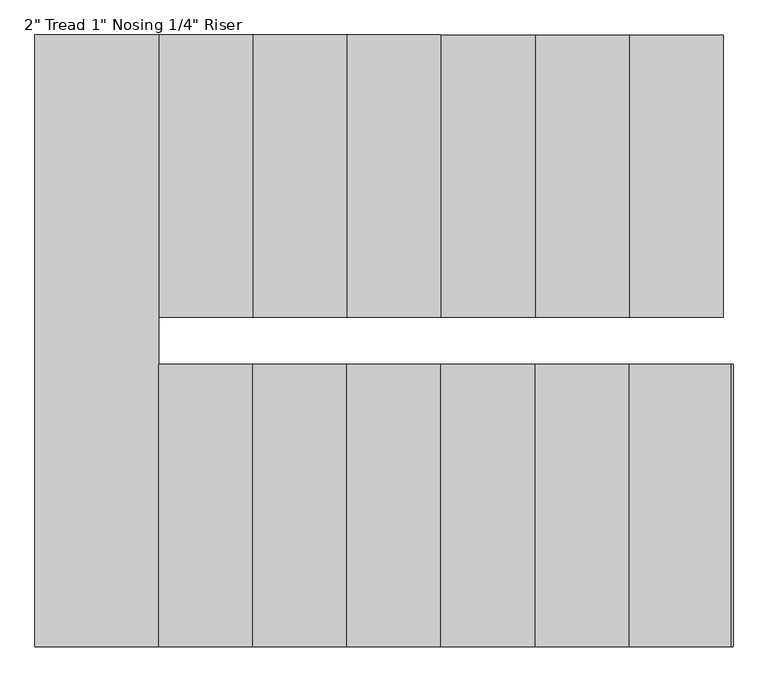
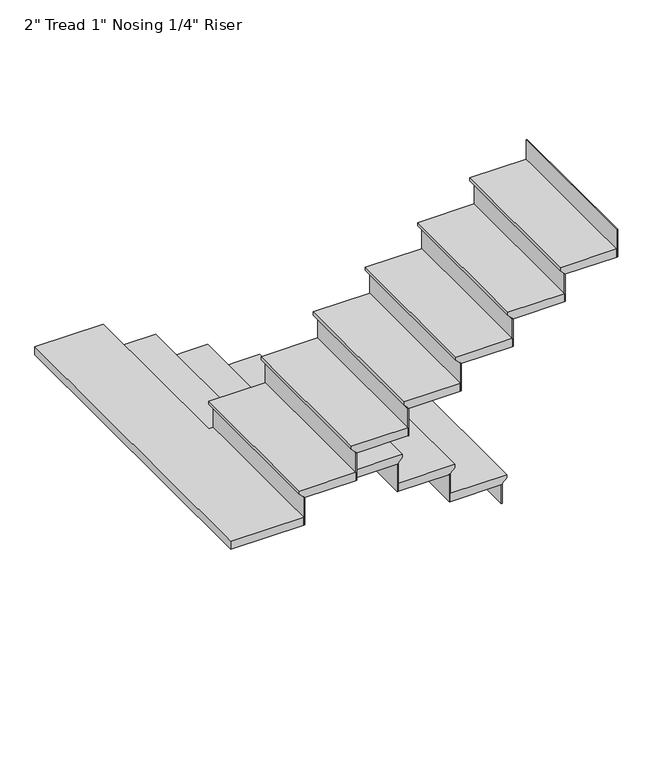
"""IFC4 building model written with IfcOpenShell, lengths in millimetres: stair flight geometry."""

from ifc_helpers import new_model, si_unit, origin, place, context, project, spatial, faceted_brep, source, transform, mapped, element, save


def stair_flight_ac649a0f(model_context):
    return source(origin(), model_context, "Body", "Brep", [
        faceted_brep([(3727.9146873, 3708.4, 9294.2833333), (3727.9146873, 3708.4, 9313.3333333), (3727.9146873, 2794.0, 9313.3333333), (3727.9146873, 2794.0, 9294.2833333), (3702.5146873, 3708.4, 9268.8833333), (3702.5146873, 2794.0, 9268.8833333), (3397.7146873, 3708.4, 9313.3333333), (3397.7146873, 2794.0, 9313.3333333), (3702.5146873, 2794.0, 9262.5333333), (3397.7146873, 2794.0, 9262.5333333), (3397.7146873, 3708.4, 9262.5333333), (3702.5146873, 3708.4, 9262.5333333)], [[[0, 1, 2, 3]], [[4, 0, 3, 5]], [[2, 1, 6, 7]], [[8, 9, 10, 11]], [[2, 7, 9, 8, 5, 3]], [[8, 11, 4, 5]], [[6, 1, 0, 4, 11, 10]], [[7, 6, 10, 9]]]),
        faceted_brep([(3702.5146873, 3708.4, 9262.5333333), (3702.5146873, 3708.4, 9144.0), (3696.1646873, 3708.4, 9144.0), (3696.1646873, 3708.4, 9262.5333333), (3702.5146873, 2794.0, 9262.5333333), (3696.1646873, 2794.0, 9262.5333333), (3696.1646873, 2794.0, 9144.0), (3702.5146873, 2794.0, 9144.0)], [[[0, 1, 2, 3]], [[4, 5, 6, 7]], [[1, 0, 4, 7]], [[2, 1, 7, 6]], [[3, 2, 6, 5]], [[0, 3, 5, 4]]]),
        faceted_brep([(3397.7146873, 3708.4, 9431.8666667), (3397.7146873, 3708.4, 9262.5333333), (3391.3646873, 3708.4, 9262.5333333), (3391.3646873, 3708.4, 9431.8666667), (3397.7146873, 2794.0, 9431.8666667), (3391.3646873, 2794.0, 9431.8666667), (3391.3646873, 2794.0, 9262.5333333), (3397.7146873, 2794.0, 9262.5333333)], [[[0, 1, 2, 3]], [[4, 5, 6, 7]], [[1, 0, 4, 7]], [[2, 1, 7, 6]], [[3, 2, 6, 5]], [[0, 3, 5, 4]]]),
        faceted_brep([(3423.1146873, 2794.0, 9482.6666667), (3423.1146873, 3708.4, 9482.6666667), (3092.9146873, 3708.4, 9482.6666667), (3092.9146873, 2794.0, 9482.6666667), (3397.7146873, 2794.0, 9431.8666667), (3092.9146873, 2794.0, 9431.8666667), (3092.9146873, 3708.4, 9431.8666667), (3397.7146873, 3708.4, 9431.8666667), (3397.7146873, 2794.0, 9438.2166667), (3423.1146873, 2794.0, 9463.6166667), (3397.7146873, 3708.4, 9438.2166667), (3423.1146873, 3708.4, 9463.6166667)], [[[0, 1, 2, 3]], [[4, 5, 6, 7]], [[0, 3, 5, 4, 8, 9]], [[4, 7, 10, 8]], [[2, 1, 11, 10, 7, 6]], [[3, 2, 6, 5]], [[11, 1, 0, 9]], [[10, 11, 9, 8]]]),
        faceted_brep([(3092.9146873, 3708.4, 9601.2), (3092.9146873, 3708.4, 9431.8666667), (3086.5646873, 3708.4, 9431.8666667), (3086.5646873, 3708.4, 9601.2), (3092.9146873, 2794.0, 9601.2), (3086.5646873, 2794.0, 9601.2), (3086.5646873, 2794.0, 9431.8666667), (3092.9146873, 2794.0, 9431.8666667)], [[[0, 1, 2, 3]], [[4, 5, 6, 7]], [[1, 0, 4, 7]], [[2, 1, 7, 6]], [[3, 2, 6, 5]], [[0, 3, 5, 4]]]),
        faceted_brep([(3118.3146873, 2794.0, 9652.0), (3118.3146873, 3708.4, 9652.0), (2788.1146873, 3708.4, 9652.0), (2788.1146873, 2794.0, 9652.0), (3092.9146873, 2794.0, 9601.2), (2788.1146873, 2794.0, 9601.2), (2788.1146873, 3708.4, 9601.2), (3092.9146873, 3708.4, 9601.2), (3092.9146873, 2794.0, 9607.55), (3118.3146873, 2794.0, 9632.95), (3092.9146873, 3708.4, 9607.55), (3118.3146873, 3708.4, 9632.95)], [[[0, 1, 2, 3]], [[4, 5, 6, 7]], [[0, 3, 5, 4, 8, 9]], [[4, 7, 10, 8]], [[2, 1, 11, 10, 7, 6]], [[3, 2, 6, 5]], [[11, 1, 0, 9]], [[10, 11, 9, 8]]]),
        faceted_brep([(2788.1146873, 3708.4, 9770.5333333), (2788.1146873, 3708.4, 9601.2), (2781.7646873, 3708.4, 9601.2), (2781.7646873, 3708.4, 9770.5333333), (2788.1146873, 2794.0, 9770.5333333), (2781.7646873, 2794.0, 9770.5333333), (2781.7646873, 2794.0, 9601.2), (2788.1146873, 2794.0, 9601.2)], [[[0, 1, 2, 3]], [[4, 5, 6, 7]], [[1, 0, 4, 7]], [[2, 1, 7, 6]], [[3, 2, 6, 5]], [[0, 3, 5, 4]]]),
        faceted_brep([(2813.5146873, 2794.0, 9821.3333333), (2813.5146873, 3708.4, 9821.3333333), (2483.3146873, 3708.4, 9821.3333333), (2483.3146873, 2794.0, 9821.3333333), (2788.1146873, 2794.0, 9770.5333333), (2483.3146873, 2794.0, 9770.5333333), (2483.3146873, 3708.4, 9770.5333333), (2788.1146873, 3708.4, 9770.5333333), (2788.1146873, 2794.0, 9776.8833333), (2813.5146873, 2794.0, 9802.2833333), (2788.1146873, 3708.4, 9776.8833333), (2813.5146873, 3708.4, 9802.2833333)], [[[0, 1, 2, 3]], [[4, 5, 6, 7]], [[0, 3, 5, 4, 8, 9]], [[4, 7, 10, 8]], [[2, 1, 11, 10, 7, 6]], [[3, 2, 6, 5]], [[11, 1, 0, 9]], [[10, 11, 9, 8]]]),
        faceted_brep([(2483.3146873, 3708.4, 9939.8666667), (2483.3146873, 3708.4, 9770.5333333), (2476.9646873, 3708.4, 9770.5333333), (2476.9646873, 3708.4, 9939.8666667), (2483.3146873, 2794.0, 9939.8666667), (2476.9646873, 2794.0, 9939.8666667), (2476.9646873, 2794.0, 9770.5333333), (2483.3146873, 2794.0, 9770.5333333)], [[[0, 1, 2, 3]], [[4, 5, 6, 7]], [[1, 0, 4, 7]], [[2, 1, 7, 6]], [[3, 2, 6, 5]], [[0, 3, 5, 4]]]),
        faceted_brep([(2508.7146873, 2794.0, 9990.6666667), (2508.7146873, 3708.4, 9990.6666667), (2178.5146873, 3708.4, 9990.6666667), (2178.5146873, 2794.0, 9990.6666667), (2483.3146873, 2794.0, 9939.8666667), (2178.5146873, 2794.0, 9939.8666667), (2178.5146873, 3708.4, 9939.8666667), (2483.3146873, 3708.4, 9939.8666667), (2483.3146873, 2794.0, 9946.2166667), (2508.7146873, 2794.0, 9971.6166667), (2483.3146873, 3708.4, 9946.2166667), (2508.7146873, 3708.4, 9971.6166667)], [[[0, 1, 2, 3]], [[4, 5, 6, 7]], [[0, 3, 5, 4, 8, 9]], [[4, 7, 10, 8]], [[2, 1, 11, 10, 7, 6]], [[3, 2, 6, 5]], [[11, 1, 0, 9]], [[10, 11, 9, 8]]]),
        faceted_brep([(2178.5146873, 3708.4, 10109.2), (2178.5146873, 3708.4, 9939.8666667), (2172.1646873, 3708.4, 9939.8666667), (2172.1646873, 3708.4, 10109.2), (2178.5146873, 2794.0, 10109.2), (2172.1646873, 2794.0, 10109.2), (2172.1646873, 2794.0, 9939.8666667), (2178.5146873, 2794.0, 9939.8666667)], [[[0, 1, 2, 3]], [[4, 5, 6, 7]], [[1, 0, 4, 7]], [[2, 1, 7, 6]], [[3, 2, 6, 5]], [[0, 3, 5, 4]]]),
        faceted_brep([(2203.9146873, 2794.0, 10160.0), (2203.9146873, 3708.4, 10160.0), (1873.7146873, 3708.4, 10160.0), (1873.7146873, 2794.0, 10160.0), (2178.5146873, 2794.0, 10109.2), (1873.7146873, 2794.0, 10109.2), (1873.7146873, 3708.4, 10109.2), (2178.5146873, 3708.4, 10109.2), (2178.5146873, 2794.0, 10115.55), (2203.9146873, 2794.0, 10140.95), (2178.5146873, 3708.4, 10115.55), (2203.9146873, 3708.4, 10140.95)], [[[0, 1, 2, 3]], [[4, 5, 6, 7]], [[0, 3, 5, 4, 8, 9]], [[4, 7, 10, 8]], [[2, 1, 11, 10, 7, 6]], [[3, 2, 6, 5]], [[11, 1, 0, 9]], [[10, 11, 9, 8]]]),
        faceted_brep([(1873.7146873, 3708.4, 10278.5333333), (1873.7146873, 3708.4, 10109.2), (1867.3646873, 3708.4, 10109.2), (1867.3646873, 3708.4, 10278.5333333), (1873.7146873, 2794.0, 10278.5333333), (1867.3646873, 2794.0, 10278.5333333), (1867.3646873, 2794.0, 10109.2), (1873.7146873, 2794.0, 10109.2)], [[[0, 1, 2, 3]], [[4, 5, 6, 7]], [[1, 0, 4, 7]], [[2, 1, 7, 6]], [[3, 2, 6, 5]], [[0, 3, 5, 4]]]),
        faceted_brep([(1924.5146873, 2641.6, 10329.3333333), (1899.1146873, 2641.6, 10329.3333333), (1899.1146873, 3708.4, 10329.3333333), (1498.6, 3708.4, 10329.3333333), (1498.6, 1727.2, 10329.3333333), (1924.5146873, 1727.2, 10329.3333333), (1899.1146873, 2641.6, 10278.5333333), (1924.5146873, 2641.6, 10278.5333333), (1924.5146873, 1727.2, 10278.5333333), (1498.6, 1727.2, 10278.5333333), (1498.6, 3708.4, 10278.5333333), (1873.7146873, 3708.4, 10278.5333333), (1873.7146873, 2794.0, 10278.5333333), (1899.1146873, 2794.0, 10278.5333333), (1899.1146873, 2794.0, 10310.2833333), (1899.1146873, 3708.4, 10310.2833333), (1873.7146873, 2794.0, 10284.8833333), (1873.7146873, 3708.4, 10284.8833333)], [[[0, 1, 2, 3, 4, 5]], [[6, 7, 8, 9, 10, 11, 12, 13]], [[1, 0, 7, 6]], [[2, 1, 6, 13, 14, 15]], [[13, 12, 16, 14]], [[12, 11, 17, 16]], [[3, 2, 15, 17, 11, 10]], [[4, 3, 10, 9]], [[5, 4, 9, 8]], [[0, 5, 8, 7]], [[17, 15, 14, 16]]]),
        faceted_brep([(1924.5146873, 1727.2, 10447.8666667), (1924.5146873, 1727.2, 10278.5333333), (1930.8646873, 1727.2, 10278.5333333), (1930.8646873, 1727.2, 10447.8666667), (1924.5146873, 2641.6, 10447.8666667), (1930.8646873, 2641.6, 10447.8666667), (1930.8646873, 2641.6, 10278.5333333), (1924.5146873, 2641.6, 10278.5333333)], [[[0, 1, 2, 3]], [[4, 5, 6, 7]], [[1, 0, 4, 7]], [[2, 1, 7, 6]], [[3, 2, 6, 5]], [[0, 3, 5, 4]]]),
        faceted_brep([(1899.1146873, 2641.6, 10498.6666667), (1899.1146873, 1727.2, 10498.6666667), (2229.3146873, 1727.2, 10498.6666667), (2229.3146873, 2641.6, 10498.6666667), (1924.5146873, 2641.6, 10447.8666667), (2229.3146873, 2641.6, 10447.8666667), (2229.3146873, 1727.2, 10447.8666667), (1924.5146873, 1727.2, 10447.8666667), (1924.5146873, 2641.6, 10454.2166667), (1899.1146873, 2641.6, 10479.6166667), (1924.5146873, 1727.2, 10454.2166667), (1899.1146873, 1727.2, 10479.6166667)], [[[0, 1, 2, 3]], [[4, 5, 6, 7]], [[0, 3, 5, 4, 8, 9]], [[4, 7, 10, 8]], [[2, 1, 11, 10, 7, 6]], [[3, 2, 6, 5]], [[11, 1, 0, 9]], [[10, 11, 9, 8]]]),
        faceted_brep([(2229.3146873, 1727.2, 10617.2), (2229.3146873, 1727.2, 10447.8666667), (2235.6646873, 1727.2, 10447.8666667), (2235.6646873, 1727.2, 10617.2), (2229.3146873, 2641.6, 10617.2), (2235.6646873, 2641.6, 10617.2), (2235.6646873, 2641.6, 10447.8666667), (2229.3146873, 2641.6, 10447.8666667)], [[[0, 1, 2, 3]], [[4, 5, 6, 7]], [[1, 0, 4, 7]], [[2, 1, 7, 6]], [[3, 2, 6, 5]], [[0, 3, 5, 4]]]),
        faceted_brep([(2203.9146873, 2641.6, 10668.0), (2203.9146873, 1727.2, 10668.0), (2534.1146873, 1727.2, 10668.0), (2534.1146873, 2641.6, 10668.0), (2229.3146873, 2641.6, 10617.2), (2534.1146873, 2641.6, 10617.2), (2534.1146873, 1727.2, 10617.2), (2229.3146873, 1727.2, 10617.2), (2229.3146873, 2641.6, 10623.55), (2203.9146873, 2641.6, 10648.95), (2229.3146873, 1727.2, 10623.55), (2203.9146873, 1727.2, 10648.95)], [[[0, 1, 2, 3]], [[4, 5, 6, 7]], [[0, 3, 5, 4, 8, 9]], [[4, 7, 10, 8]], [[2, 1, 11, 10, 7, 6]], [[3, 2, 6, 5]], [[11, 1, 0, 9]], [[10, 11, 9, 8]]]),
        faceted_brep([(2534.1146873, 1727.2, 10786.5333333), (2534.1146873, 1727.2, 10617.2), (2540.4646873, 1727.2, 10617.2), (2540.4646873, 1727.2, 10786.5333333), (2534.1146873, 2641.6, 10786.5333333), (2540.4646873, 2641.6, 10786.5333333), (2540.4646873, 2641.6, 10617.2), (2534.1146873, 2641.6, 10617.2)], [[[0, 1, 2, 3]], [[4, 5, 6, 7]], [[1, 0, 4, 7]], [[2, 1, 7, 6]], [[3, 2, 6, 5]], [[0, 3, 5, 4]]]),
        faceted_brep([(2508.7146873, 2641.6, 10837.3333333), (2508.7146873, 1727.2, 10837.3333333), (2838.9146873, 1727.2, 10837.3333333), (2838.9146873, 2641.6, 10837.3333333), (2534.1146873, 2641.6, 10786.5333333), (2838.9146873, 2641.6, 10786.5333333), (2838.9146873, 1727.2, 10786.5333333), (2534.1146873, 1727.2, 10786.5333333), (2534.1146873, 2641.6, 10792.8833333), (2508.7146873, 2641.6, 10818.2833333), (2534.1146873, 1727.2, 10792.8833333), (2508.7146873, 1727.2, 10818.2833333)], [[[0, 1, 2, 3]], [[4, 5, 6, 7]], [[0, 3, 5, 4, 8, 9]], [[4, 7, 10, 8]], [[2, 1, 11, 10, 7, 6]], [[3, 2, 6, 5]], [[11, 1, 0, 9]], [[10, 11, 9, 8]]]),
        faceted_brep([(2838.9146873, 1727.2, 10955.8666667), (2838.9146873, 1727.2, 10786.5333333), (2845.2646873, 1727.2, 10786.5333333), (2845.2646873, 1727.2, 10955.8666667), (2838.9146873, 2641.6, 10955.8666667), (2845.2646873, 2641.6, 10955.8666667), (2845.2646873, 2641.6, 10786.5333333), (2838.9146873, 2641.6, 10786.5333333)], [[[0, 1, 2, 3]], [[4, 5, 6, 7]], [[1, 0, 4, 7]], [[2, 1, 7, 6]], [[3, 2, 6, 5]], [[0, 3, 5, 4]]]),
        faceted_brep([(2813.5146873, 2641.6, 11006.6666667), (2813.5146873, 1727.2, 11006.6666667), (3143.7146873, 1727.2, 11006.6666667), (3143.7146873, 2641.6, 11006.6666667), (2838.9146873, 2641.6, 10955.8666667), (3143.7146873, 2641.6, 10955.8666667), (3143.7146873, 1727.2, 10955.8666667), (2838.9146873, 1727.2, 10955.8666667), (2838.9146873, 2641.6, 10962.2166667), (2813.5146873, 2641.6, 10987.6166667), (2838.9146873, 1727.2, 10962.2166667), (2813.5146873, 1727.2, 10987.6166667)], [[[0, 1, 2, 3]], [[4, 5, 6, 7]], [[0, 3, 5, 4, 8, 9]], [[4, 7, 10, 8]], [[2, 1, 11, 10, 7, 6]], [[3, 2, 6, 5]], [[11, 1, 0, 9]], [[10, 11, 9, 8]]]),
        faceted_brep([(3143.7146873, 1727.2, 11125.2), (3143.7146873, 1727.2, 10955.8666667), (3150.0646873, 1727.2, 10955.8666667), (3150.0646873, 1727.2, 11125.2), (3143.7146873, 2641.6, 11125.2), (3150.0646873, 2641.6, 11125.2), (3150.0646873, 2641.6, 10955.8666667), (3143.7146873, 2641.6, 10955.8666667)], [[[0, 1, 2, 3]], [[4, 5, 6, 7]], [[1, 0, 4, 7]], [[2, 1, 7, 6]], [[3, 2, 6, 5]], [[0, 3, 5, 4]]]),
        faceted_brep([(3118.3146873, 2641.6, 11176.0), (3118.3146873, 1727.2, 11176.0), (3448.5146873, 1727.2, 11176.0), (3448.5146873, 2641.6, 11176.0), (3143.7146873, 2641.6, 11125.2), (3448.5146873, 2641.6, 11125.2), (3448.5146873, 1727.2, 11125.2), (3143.7146873, 1727.2, 11125.2), (3143.7146873, 2641.6, 11131.55), (3118.3146873, 2641.6, 11156.95), (3143.7146873, 1727.2, 11131.55), (3118.3146873, 1727.2, 11156.95)], [[[0, 1, 2, 3]], [[4, 5, 6, 7]], [[0, 3, 5, 4, 8, 9]], [[4, 7, 10, 8]], [[2, 1, 11, 10, 7, 6]], [[3, 2, 6, 5]], [[11, 1, 0, 9]], [[10, 11, 9, 8]]]),
        faceted_brep([(3448.5146873, 1727.2, 11294.5333333), (3448.5146873, 1727.2, 11125.2), (3454.8646873, 1727.2, 11125.2), (3454.8646873, 1727.2, 11294.5333333), (3448.5146873, 2641.6, 11294.5333333), (3454.8646873, 2641.6, 11294.5333333), (3454.8646873, 2641.6, 11125.2), (3448.5146873, 2641.6, 11125.2)], [[[0, 1, 2, 3]], [[4, 5, 6, 7]], [[1, 0, 4, 7]], [[2, 1, 7, 6]], [[3, 2, 6, 5]], [[0, 3, 5, 4]]]),
        faceted_brep([(3753.3146873, 1727.2, 11463.8666667), (3753.3146873, 1727.2, 11294.5333333), (3759.6646873, 1727.2, 11294.5333333), (3759.6646873, 1727.2, 11463.8666667), (3753.3146873, 2641.6, 11463.8666667), (3759.6646873, 2641.6, 11463.8666667), (3759.6646873, 2641.6, 11294.5333333), (3753.3146873, 2641.6, 11294.5333333)], [[[0, 1, 2, 3]], [[4, 5, 6, 7]], [[1, 0, 4, 7]], [[2, 1, 7, 6]], [[3, 2, 6, 5]], [[0, 3, 5, 4]]]),
        faceted_brep([(3423.1146873, 2641.6, 11345.3333333), (3423.1146873, 1727.2, 11345.3333333), (3753.3146873, 1727.2, 11345.3333333), (3753.3146873, 2641.6, 11345.3333333), (3448.5146873, 2641.6, 11294.5333333), (3753.3146873, 2641.6, 11294.5333333), (3753.3146873, 1727.2, 11294.5333333), (3448.5146873, 1727.2, 11294.5333333), (3448.5146873, 2641.6, 11300.8833333), (3423.1146873, 2641.6, 11326.2833333), (3448.5146873, 1727.2, 11300.8833333), (3423.1146873, 1727.2, 11326.2833333)], [[[0, 1, 2, 3]], [[4, 5, 6, 7]], [[0, 3, 5, 4, 8, 9]], [[4, 7, 10, 8]], [[2, 1, 11, 10, 7, 6]], [[3, 2, 6, 5]], [[11, 1, 0, 9]], [[10, 11, 9, 8]]]),
    ])


if __name__ == "__main__":
    model = new_model("IFC4")
    model_context = context("Model", 3, world=origin())
    ifc_project = project(units=[si_unit("LENGTHUNIT", "METRE", prefix="MILLI")], contexts=[model_context])
    site = spatial("IfcSite", under=ifc_project)
    building = spatial("IfcBuilding", under=site)
    placement = place(None, origin())
    stair_flight_shape = stair_flight_ac649a0f(model_context)
    element("IfcStairFlight", 1, ObjectType="2\" Tread 1\" Nosing 1/4\" Riser", at=placement, inside=building, context=model_context, shape_type="MappedRepresentation", body=[
        mapped(stair_flight_shape, transform((0.0, 0.0, 0.0), x_axis=(1.0, 0.0, 0.0), y_axis=(0.0, 1.0, 0.0), z_axis=(0.0, 0.0, 1.0))),
    ])
    save(model, "model.ifc")
